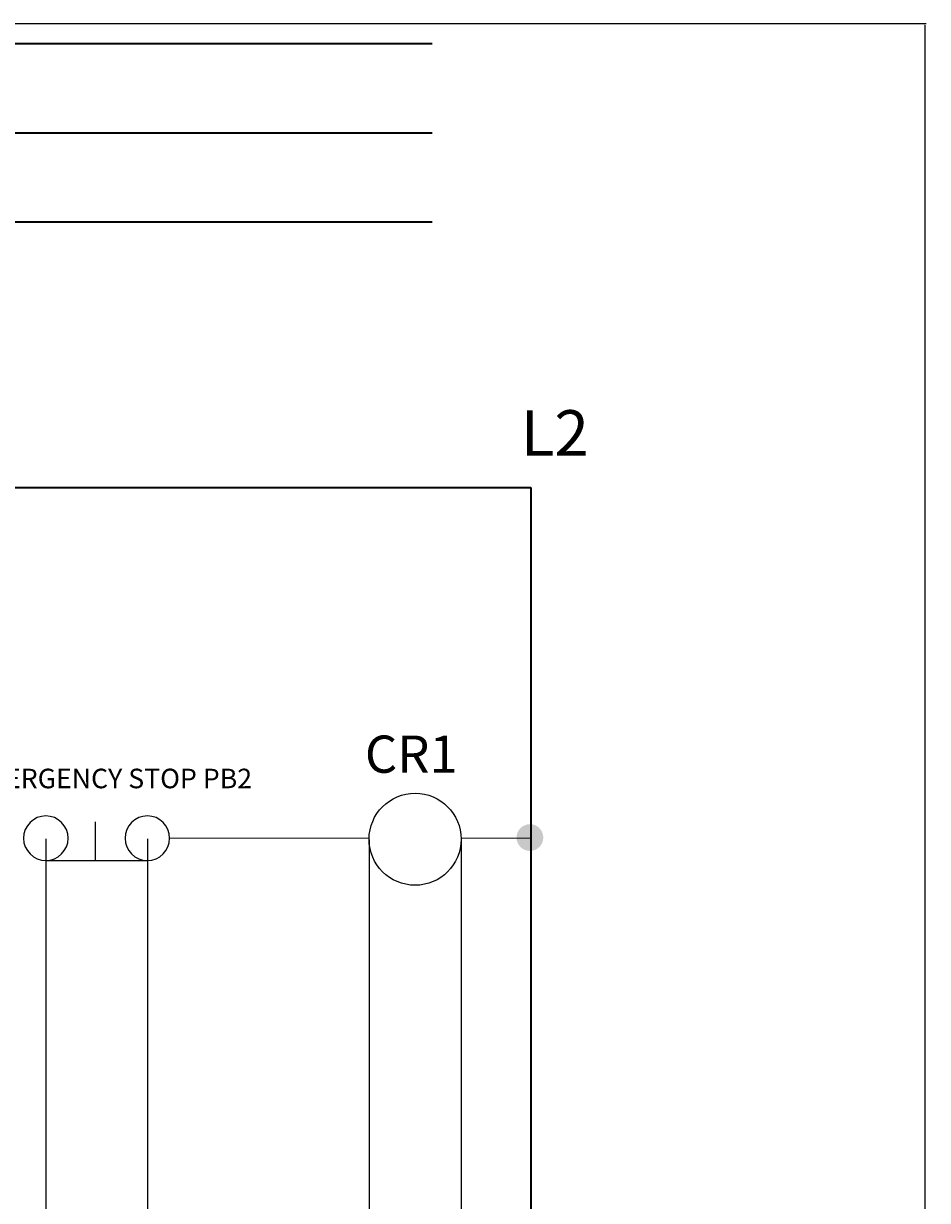
# Model space of a CAD drawing. Units: inches. Extents: x 738 to 1068, y 378 to 757.
# Tile 41 of 41: x 967 to 1068, y 606 to 738. Entities that reach past the tile are written whole.
import ezdxf

# ---------------------------------------------------------------- set-up
doc = ezdxf.new("R2010")
doc.units = ezdxf.units.IN
doc.header["$MEASUREMENT"] = 0
for name, color, linetype, lineweight in [('A-ANNO-DIMS', 2, 'Continuous', 18), ('E-ANNO-TEXT', 7, 'Continuous', 18), ('E-CONN-PATT', 7, 'Continuous', 13), ('E-CTRL-COIL', 4, 'Continuous', 25), ('E-CTRL-PBTN', 4, 'Continuous', 25), ('E-CTRL-WIRE', 7, 'Continuous', 18), ('E-POWR-FEED', 7, 'Continuous', 35)]:
    doc.layers.add(name, color=color, linetype=linetype, lineweight=lineweight)
doc.styles.get("Standard").update_dxf_attribs({"font": 'arial.ttf'})
doc.dimstyles.get("Standard").update_dxf_attribs({"dimtxt": 0.18, "dimasz": 0.18, "dimexe": 0.18, "dimexo": 0.0625, "dimgap": 0.09, "dimtad": 0, "dimtih": 1, "dimtoh": 1, "dimdec": 4, "dimzin": 0, "dimdsep": 46, "dimtxsty": 'Standard', "dimcen": 0.09, "dimadec": 0, "dimazin": 0, "dimtfac": 1, "dimtdec": 4, "dimtofl": 0, "dimtmove": 0, "dimatfit": 3, "dimfxl": 1, "dimtolj": 1, "dimtzin": 0, "dimarcsym": 0})

# ---------------------------------------------------------------- blocks, each defined once
blk = doc.blocks.new('RELAY-COIL')
blk.add_circle((5.16, 5.16), 5.16)
blk = doc.blocks.new('*D18')
at = {"layer": 'A-ANNO-DIMS', "color": 0, "lineweight": -2, "transparency": 16777216}
for p, q in [((901.52, 738.38), (1068.18, 738.38)), ((1068, 738.2), (1068, 569.17)), ((1068, 399.78), (1068, 568.8)), ((1023.84, 399.6), (1068.18, 399.6))]:
    blk.add_line(p, q, dxfattribs=at)
at = {"layer": 'A-ANNO-DIMS', "color": 0, "transparency": 16777216}
for points in [[(1067.97, 738.2), (1068.03, 738.2), (1068, 738.38)], [(1067.97, 399.78), (1068.03, 399.78), (1068, 399.6)]]:
    blk.add_solid(points, dxfattribs=at)
at = {"layer": 'Defpoints', "color": 0, "transparency": 16777216}
for p in [(901.46, 738.38), (1068, 738.38), (1023.78, 399.6)]:
    blk.add_point(p, dxfattribs=at)
at = {"layer": 'A-ANNO-DIMS', "color": 0, "transparency": 16777216, "insert": (1068, 568.99), "char_height": 0.18, "attachment_point": 5}
blk.add_mtext('\\A1;338.8', dxfattribs=at)
blk = doc.blocks.new('*D28')
at = {"layer": 'A-ANNO-DIMS', "color": 0, "lineweight": -2, "transparency": 16777216}
for p, q in [((923.51, 646.92), (923.51, 378.24)), ((969.44, 646.92), (969.44, 378.24)), ((923.69, 378.42), (946.08, 378.42)), ((969.26, 378.42), (946.87, 378.42))]:
    blk.add_line(p, q, dxfattribs=at)
at = {"layer": 'A-ANNO-DIMS', "color": 0, "transparency": 16777216}
for points in [[(923.69, 378.45), (923.69, 378.39), (923.51, 378.42)], [(969.26, 378.45), (969.26, 378.39), (969.44, 378.42)]]:
    blk.add_solid(points, dxfattribs=at)
at = {"layer": 'Defpoints', "color": 0, "transparency": 16777216}
for p in [(923.51, 646.99), (969.44, 646.99), (969.44, 378.42)]:
    blk.add_point(p, dxfattribs=at)
at = {"layer": 'A-ANNO-DIMS', "color": 0, "transparency": 16777216, "insert": (946.48, 378.42), "char_height": 0.18, "attachment_point": 5}
blk.add_mtext('\\A1;45.93', dxfattribs=at)
blk = doc.blocks.new('*D29')
at = {"layer": 'A-ANNO-DIMS', "color": 0, "lineweight": -2, "transparency": 16777216}
for p, q in [((980.83, 646.92), (980.83, 378.24)), ((1005.69, 646.81), (1005.69, 378.24)), ((981.01, 378.42), (992.79, 378.42)), ((1005.51, 378.42), (993.72, 378.42))]:
    blk.add_line(p, q, dxfattribs=at)
at = {"layer": 'A-ANNO-DIMS', "color": 0, "transparency": 16777216}
for points in [[(981.01, 378.45), (981.01, 378.39), (980.83, 378.42)], [(1005.51, 378.45), (1005.51, 378.39), (1005.69, 378.42)]]:
    blk.add_solid(points, dxfattribs=at)
at = {"layer": 'Defpoints', "color": 0, "transparency": 16777216}
for p in [(980.83, 646.99), (1005.69, 646.87), (1005.69, 378.42)]:
    blk.add_point(p, dxfattribs=at)
at = {"layer": 'A-ANNO-DIMS', "color": 0, "transparency": 16777216, "insert": (993.26, 378.42), "char_height": 0.18, "attachment_point": 5}
blk.add_mtext('\\A1;24.864', dxfattribs=at)
blk = doc.blocks.new('*D30')
at = {"layer": 'A-ANNO-DIMS', "color": 0, "lineweight": -2, "transparency": 16777216}
for p, q in [((1016.01, 646.81), (1016.01, 378.24)), ((1023.82, 646.92), (1023.82, 378.24)), ((1016.19, 378.42), (1019.54, 378.42)), ((1023.64, 378.42), (1020.29, 378.42))]:
    blk.add_line(p, q, dxfattribs=at)
at = {"layer": 'A-ANNO-DIMS', "color": 0, "transparency": 16777216}
for points in [[(1016.19, 378.45), (1016.19, 378.39), (1016.01, 378.42)], [(1023.64, 378.45), (1023.64, 378.39), (1023.82, 378.42)]]:
    blk.add_solid(points, dxfattribs=at)
at = {"layer": 'Defpoints', "color": 0, "transparency": 16777216}
for p in [(1023.82, 646.99), (1016.01, 646.87), (1023.82, 378.42)]:
    blk.add_point(p, dxfattribs=at)
at = {"layer": 'A-ANNO-DIMS', "color": 0, "transparency": 16777216, "insert": (1019.92, 378.42), "char_height": 0.18, "attachment_point": 5}
blk.add_mtext('\\A1;7.811', dxfattribs=at)

msp = doc.modelspace()

# ---------------------------------------------------------------- hatches: boundary and pattern name
at = {"layer": 'E-CONN-PATT'}
h = msp.add_hatch(color=256, dxfattribs=at)
h.dxf.hatch_style = 1
h.paths.add_polyline_path([(1025.2273, 647.0567, 1), (1022.2273, 647.0567, 1)])

# ---------------------------------------------------------------- linework, layer by layer
at = {"layer": 'E-CTRL-PBTN'}
for p, q in [((975.0261, 644.5269), (975.0261, 648.8389)), ((969.4395, 644.4853), (980.8252, 644.4853))]:
    msp.add_line(p, q, dxfattribs=at)
for points in [[(966.9395, 646.9853, 1), (971.9395, 646.9853, 1)], [(978.3252, 646.9853, 1), (983.3252, 646.9853, 1)]]:
    msp.add_lwpolyline(points, format="xyb", close=True, dxfattribs=at)
at = {"layer": 'E-CTRL-WIRE'}
for p, q in [((983.3252, 646.9853), (1005.6909, 646.9853)), ((1016.0116, 646.9853), (1023.824, 646.9853))]:
    msp.add_line(p, q, dxfattribs=at)
at = {"layer": 'E-POWR-FEED'}
for p, q in [((841.9816, 736.1282), (1012.7462, 736.1282)), ((841.9816, 726.1282), (1012.7462, 726.1282)), ((841.9816, 716.1282), (1012.7462, 716.1282)), ((953.0038, 686.3292), (1023.824, 686.3292)), ((1023.824, 686.3292), (1023.824, 431.3208))]:
    msp.add_line(p, q, dxfattribs=at)

# ---------------------------------------------------------------- block references
at = {"layer": 'E-CTRL-COIL'}
msp.add_blockref('RELAY-COIL', (1005.69, 641.707), dxfattribs=at)

# ---------------------------------------------------------------- texts
at = {"layer": 'E-ANNO-TEXT'}
for s, height, p in [('L2', 5.11096, (1022.6866, 689.8867)), ('CR1', 4.17507, (1005.2185, 654.3262)), ('EMERGENCY STOP PB2', 2.19392, (960.6679, 652.5875))]:
    msp.add_text(s, height=height, dxfattribs=at).set_placement(p)

# ---------------------------------------------------------------- dimensions: what is measured, and where the dimension line sits
at = {"layer": 'A-ANNO-DIMS'}
dim = msp.add_linear_dim(base=(1067.9992, 738.3751), p1=(1023.779, 399.5952), p2=(901.4622, 738.3751), angle=90, dimstyle='Standard', override={"dimdec": 1, "dimlfac": 1, "dimrnd": 0, "dimzin": 0, "dimdsep": 46, "dimlunit": 2}, dxfattribs=at)
dim.commit()
dim.dimension.update_dxf_attribs({"geometry": '*D18', "text_midpoint": (1067.9992, 568.9851)})
for base, p1, p2, override, picture, middle in [((969.4395, 378.4191), (923.5105, 646.9853), (969.4395, 646.9853), {"dimdec": 2, "dimlfac": 1, "dimrnd": 0, "dimzin": 0, "dimdsep": 46, "dimlunit": 2}, '*D28', (946.475, 378.4191)), ((1005.6896, 378.4191), (980.8252, 646.9853), (1005.6896, 646.8683), {"dimdec": 3, "dimlfac": 1, "dimrnd": 0, "dimzin": 0, "dimdsep": 46, "dimlunit": 2}, '*D29', (993.2574, 378.4191)), ((1023.824, 378.4191), (1016.0129, 646.8683), (1023.824, 646.9853), {"dimdec": 3, "dimlfac": 1, "dimrnd": 0, "dimzin": 0, "dimdsep": 46, "dimlunit": 2}, '*D30', (1019.9185, 378.4191))]:
    dim = msp.add_linear_dim(base=base, p1=p1, p2=p2, dimstyle='Standard', override=override, dxfattribs=at)
    dim.commit()
    dim.dimension.update_dxf_attribs({"geometry": picture, "text_midpoint": middle})

doc.saveas('drawing.dxf')
